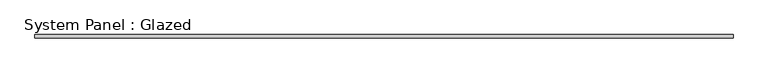
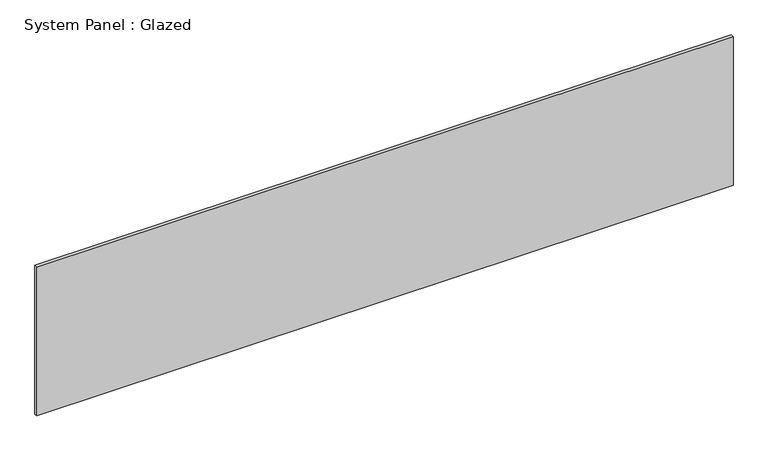
"""IFC4 building model written with IfcOpenShell, lengths in millimetres: plate geometry, System Panel : Glazed."""

from ifc_helpers import new_model, si_unit, origin, origin_with_axes, place, context, project, spatial, polyline, outline, extrude, source, transform, mapped, element, save


def system_panel_glazed_aff0b4bd(model_context):
    return source(origin(), model_context, "Body", "SweptSolid", [
        extrude(outline(polyline([(2676.525, 19.05), (-2676.525, 19.05), (-2676.525, 44.45), (2676.525, 44.45), (2676.525, 19.05)])), origin_with_axes(), (0.0, 0.0, 1.0), 1207.4564694),
    ])


if __name__ == "__main__":
    model = new_model("IFC4")
    model_context = context("Model", 3, world=origin())
    ifc_project = project(units=[si_unit("LENGTHUNIT", "METRE", prefix="MILLI")], contexts=[model_context])
    site = spatial("IfcSite", under=ifc_project)
    building = spatial("IfcBuilding", under=site)
    placement = place(None, origin())
    system_panel_glazed_shape = system_panel_glazed_aff0b4bd(model_context)
    element("IfcPlate", 1, ObjectType="System Panel : Glazed", at=placement, inside=building, context=model_context, shape_type="MappedRepresentation", body=[
        mapped(system_panel_glazed_shape, transform((0.0, 0.0, 0.0), x_axis=(1.0, 0.0, 0.0), y_axis=(0.0, 1.0, 0.0), z_axis=(0.0, 0.0, 1.0))),
    ])
    save(model, "model.ifc")

# Revit data of these elements
# Type "System Panel : Glazed"
#   Construction Type Id = "GSP4R"
#   Analytic Construction = "1/8 in Pilkington single glazing"
#   Visual Light Transmittance = 0.9
#   Solar Heat Gain Coefficient = 0.86
#   Heat Transfer Coefficient (U) = 1.18115 BTU/(h·ft²·°F)
#   Define Thermal Properties by = 1
# Element 1 (IfcPlate, "System Panel : Glazed")
#   Materials on its faces: "Glass"
# Materials
#   "Glass": class "Glass", colour RGB 0 128 192, transparency 0.75, Description = "Soda Lime Glass", Cost = 0
